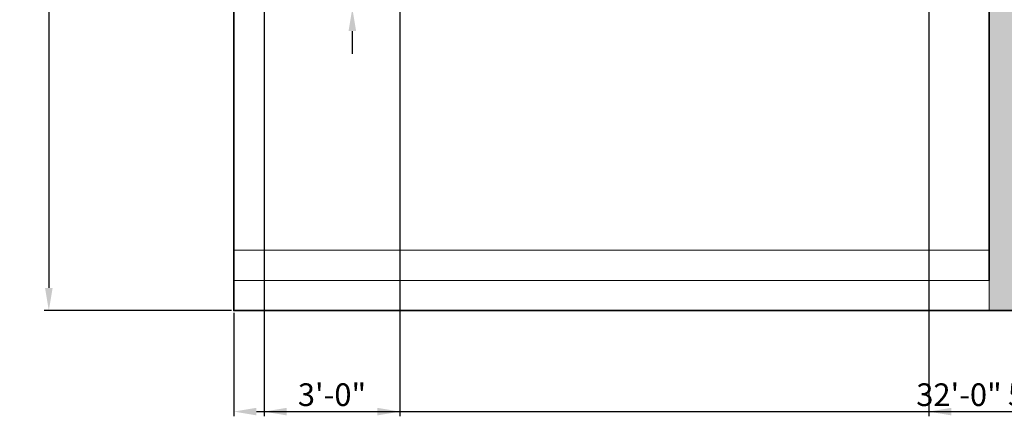
# Model space of a CAD drawing. Units: inches. Extents: x 2129 to 3258, y 1851 to 3021.
# Tile 1 of 10: x 2129 to 2390, y 1851 to 1956. Entities that reach past the tile are written whole.
import ezdxf

# ---------------------------------------------------------------- set-up
doc = ezdxf.new("R2010")
doc.units = ezdxf.units.IN
for name, color, linetype, lineweight in [('A-ANNO-DIMS', 2, 'Continuous', 18), ('A-FLOR-STRS', 7, 'Continuous', 20), ('A-WALL', 7, 'Continuous', 35)]:
    doc.layers.add(name, color=color, linetype=linetype, lineweight=lineweight)
doc.layers.add('A-WALL-PATT', color=32, linetype='Continuous', lineweight=13, true_color=0xcd6928)
doc.styles.get("Standard").update_dxf_attribs({"font": 'arial.ttf'})
doc.dimstyles.new('ISO-25', dxfattribs={"dimtxt": 6, "dimasz": 6, "dimexe": 1.25, "dimexo": 0.625, "dimtad": 1, "dimdec": 1, "dimlunit": 3, "dimtxsty": 'Standard', "dimcen": 2.5, "dimclrd": 5, "dimclre": 5, "dimadec": 0, "dimazin": 0, "dimtfac": 1, "dimtdec": 1, "dimtmove": 0, "dimatfit": 3, "dimfxl": 1, "dimarcsym": 0})

# ---------------------------------------------------------------- blocks, each defined once
blk = doc.blocks.new('*D6')
at = {"layer": 'A-ANNO-DIMS', "color": 0, "lineweight": -2, "transparency": 16777216}
for p, q in [((2185.3, 2407.23), (2135.71, 2407.23)), ((2136.96, 2401.23), (2136.96, 1885.23)), ((2185.3, 1879.23), (2135.71, 1879.23))]:
    blk.add_line(p, q, dxfattribs=at)
at = {"layer": 'A-ANNO-DIMS', "color": 0, "transparency": 16777216}
for points in [[(2135.96, 2401.23), (2137.96, 2401.23), (2136.96, 2407.23)], [(2135.96, 1885.23), (2137.96, 1885.23), (2136.96, 1879.23)]]:
    blk.add_solid(points, dxfattribs=at)
at = {"layer": 'Defpoints', "color": 0, "transparency": 16777216}
for p in [(2185.93, 2407.23), (2136.96, 1879.23), (2185.93, 1879.23)]:
    blk.add_point(p, dxfattribs=at)
at = {"layer": 'A-ANNO-DIMS', "color": 0, "transparency": 16777216, "insert": (2133.34, 2143.23), "char_height": 6, "attachment_point": 5, "rotation": 90}
blk.add_mtext("44'", dxfattribs=at)
blk = doc.blocks.new('*D63')
at = {"layer": 'A-ANNO-DIMS', "color": 5, "lineweight": -2, "transparency": 16777216}
for p, q in [((2217.31, 1973.23), (2217.31, 2017.06)), ((2221.94, 1967.23), (2216.06, 1967.23)), ((2217.31, 1959.23), (2217.31, 1967.23)), ((2221.94, 1959.23), (2216.06, 1959.23)), ((2217.31, 1953.23), (2217.31, 1947.23))]:
    blk.add_line(p, q, dxfattribs=at)
at = {"layer": 'A-ANNO-DIMS', "color": 5, "transparency": 16777216}
for points in [[(2216.31, 1973.23), (2218.31, 1973.23), (2217.31, 1967.23)], [(2216.31, 1953.23), (2218.31, 1953.23), (2217.31, 1959.23)]]:
    blk.add_solid(points, dxfattribs=at)
at = {"layer": 'Defpoints', "color": 0, "transparency": 16777216}
for p in [(2217.31, 1967.23), (2222.56, 1967.23), (2222.56, 1959.23)]:
    blk.add_point(p, dxfattribs=at)
at = {"layer": 'A-ANNO-DIMS', "color": 0, "transparency": 16777216, "insert": (2213.63, 1998.15), "char_height": 6, "attachment_point": 5, "rotation": 90}
blk.add_mtext('0\'-8" TYP.', dxfattribs=at)
blk = doc.blocks.new('*D86')
at = {"layer": 'A-ANNO-DIMS', "color": 5, "lineweight": -2, "transparency": 16777216}
for p, q in [((2185.93, 1878.61), (2185.93, 1851.23)), ((2569.93, 1878.61), (2569.93, 1851.23)), ((2191.93, 1852.48), (2563.93, 1852.48))]:
    blk.add_line(p, q, dxfattribs=at)
at = {"layer": 'A-ANNO-DIMS', "color": 5, "transparency": 16777216}
for points in [[(2191.93, 1853.48), (2191.93, 1851.48), (2185.93, 1852.48)], [(2563.93, 1853.48), (2563.93, 1851.48), (2569.93, 1852.48)]]:
    blk.add_solid(points, dxfattribs=at)
at = {"layer": 'Defpoints', "color": 0, "transparency": 16777216}
for p in [(2185.93, 1879.23), (2569.93, 1879.23), (2569.93, 1852.48)]:
    blk.add_point(p, dxfattribs=at)
at = {"layer": 'A-ANNO-DIMS', "color": 0, "transparency": 16777216, "insert": (2377.93, 1856.18), "char_height": 6, "attachment_point": 5}
blk.add_mtext('32\'-0"', dxfattribs=at)
blk = doc.blocks.new('*D91')
at = {"layer": 'A-ANNO-DIMS', "color": 5, "lineweight": -2, "transparency": 16777216}
for p, q in [((2369.93, 2314.61), (2369.93, 1851.23)), ((2429.93, 2314.61), (2429.93, 1851.23)), ((2375.93, 1852.48), (2423.93, 1852.48))]:
    blk.add_line(p, q, dxfattribs=at)
at = {"layer": 'A-ANNO-DIMS', "color": 5, "transparency": 16777216}
for points in [[(2375.93, 1853.48), (2375.93, 1851.48), (2369.93, 1852.48)], [(2423.93, 1853.48), (2423.93, 1851.48), (2429.93, 1852.48)]]:
    blk.add_solid(points, dxfattribs=at)
at = {"layer": 'Defpoints', "color": 0, "transparency": 16777216}
for p in [(2369.93, 2315.23), (2429.93, 2315.23), (2429.93, 1852.48)]:
    blk.add_point(p, dxfattribs=at)
at = {"layer": 'A-ANNO-DIMS', "color": 0, "transparency": 16777216, "insert": (2399.93, 1856.17), "char_height": 6, "attachment_point": 5}
blk.add_mtext('5\'-0"', dxfattribs=at)
blk = doc.blocks.new('*D97')
at = {"layer": 'A-ANNO-DIMS', "color": 5, "lineweight": -2, "transparency": 16777216}
for p, q in [((2193.93, 2272.48), (2193.93, 1851.23)), ((2229.93, 2272.48), (2229.93, 1851.23)), ((2199.93, 1852.48), (2223.93, 1852.48))]:
    blk.add_line(p, q, dxfattribs=at)
at = {"layer": 'A-ANNO-DIMS', "color": 5, "transparency": 16777216}
for points in [[(2199.93, 1853.48), (2199.93, 1851.48), (2193.93, 1852.48)], [(2223.93, 1853.48), (2223.93, 1851.48), (2229.93, 1852.48)]]:
    blk.add_solid(points, dxfattribs=at)
at = {"layer": 'Defpoints', "color": 0, "transparency": 16777216}
for p in [(2193.93, 2273.1), (2229.93, 2273.1), (2229.93, 1852.48)]:
    blk.add_point(p, dxfattribs=at)
at = {"layer": 'A-ANNO-DIMS', "color": 0, "transparency": 16777216, "insert": (2211.93, 1856.18), "char_height": 6, "attachment_point": 5}
blk.add_mtext('3\'-0"', dxfattribs=at)

msp = doc.modelspace()

# ---------------------------------------------------------------- hatches: boundary and pattern name
at = {"layer": 'A-WALL-PATT'}
h = msp.add_hatch(color=256, dxfattribs=at)
h.dxf.hatch_style = 1
h.paths.add_polyline_path([(2393.39, 2407.23), (2185.93, 2407.23), (2185.93, 2394.06), (2193.93, 2394.06), (2193.93, 2399.23), (2361.93, 2399.23), (2361.93, 2355.23), (2361.93, 2347.23), (2361.93, 2258.25), (2369.93, 2258.25), (2369.93, 2307.23), (2429.93, 2307.23), (2429.93, 2303.23), (2437.93, 2303.23), (2437.93, 2327.23), (2429.93, 2327.23), (2429.93, 2315.23), (2369.93, 2315.23), (2369.93, 2399.23), (2393.39, 2399.23)])
h.paths.add_polyline_path([(2569.93, 2407.23), (2410.42, 2407.23), (2410.42, 2399.23), (2429.93, 2399.23), (2429.93, 2351.23), (2437.93, 2351.23), (2437.93, 2399.23), (2561.93, 2399.23), (2561.93, 2317.22), (2569.93, 2317.22)])
h.paths.add_polyline_path([(2569.93, 2282.22), (2561.93, 2282.22), (2561.93, 2243.23), (2437.93, 2243.23), (2437.93, 2249.23), (2429.93, 2249.23), (2429.93, 2235.23), (2561.93, 2235.23), (2561.93, 2155.23), (2379.93, 2155.23), (2379.93, 2147.23), (2385.93, 2147.23), (2385.93, 2141.23), (2393.93, 2141.23), (2393.93, 2147.23), (2469.93, 2147.23), (2469.93, 2111.23), (2477.93, 2111.23), (2477.93, 2147.23), (2561.93, 2147.23), (2561.93, 2129.53), (2569.93, 2129.53)])
h.paths.add_polyline_path([(2569.93, 2112.5), (2561.93, 2112.5), (2561.93, 2063.23), (2477.93, 2063.23), (2477.93, 2069.23), (2469.93, 2069.23), (2469.93, 2063.23), (2445.93, 2063.23), (2445.93, 2055.23), (2561.93, 2055.23), (2561.93, 1951.04), (2569.93, 1951.04)])
h.paths.add_polyline_path([(2569.93, 1916.04), (2561.93, 1916.04), (2561.93, 1887.23), (2393.93, 1887.23), (2393.93, 2055.23), (2399.93, 2055.23), (2399.93, 2063.23), (2393.93, 2063.23), (2393.93, 2087.23), (2385.93, 2087.23), (2385.93, 1887.23), (2385.93, 1879.23), (2569.93, 1879.23)])
h.paths.add_polyline_path([(2193.93, 2147.23), (2289.93, 2147.23), (2289.93, 2155.23), (2193.93, 2155.23), (2193.93, 2170.77), (2185.93, 2170.77), (2185.93, 2056.85), (2193.93, 2056.85)])
h.paths.add_polyline_path([(2193.93, 2021.85), (2185.93, 2021.85), (2185.93, 1959.23), (2222.56, 1959.23), (2222.56, 1967.23), (2193.93, 1967.23)])
h.paths.add_polyline_path([(2307.93, 1967.23), (2257.56, 1967.23), (2257.56, 1959.23), (2307.93, 1959.23)])
h.paths.add_polyline_path([(2255.61, 2368.18), (2321.09, 2368.18), (2321.09, 2384.66), (2255.61, 2384.66)], flags=25)
h.paths.add_polyline_path([(2282.89, 2032.34), (2325.27, 2032.34), (2325.27, 2051.27), (2282.89, 2051.27)], flags=9)
h.paths.add_polyline_path([(2404.09, 1945.18), (2463.36, 1945.18), (2463.36, 1961.66), (2404.09, 1961.66)], flags=25)
h.paths.add_polyline_path([(2494.41, 2286.84), (2553.68, 2286.84), (2553.68, 2303.32), (2494.41, 2303.32)], flags=9)
h.paths.add_polyline_path([(2389.71, 2321.98), (2411.09, 2321.98), (2411.09, 2338.47), (2389.71, 2338.47)], flags=25)
h.paths.add_polyline_path([(2219.41, 2162.82), (2258.18, 2162.82), (2258.18, 2179.3), (2219.41, 2179.3)], flags=9)
h.paths.add_polyline_path([(2249.68, 2306.23), (2298.12, 2306.23), (2298.12, 2323.98), (2249.68, 2323.98)], flags=25)

# ---------------------------------------------------------------- linework, layer by layer
at = {"layer": 'A-FLOR-STRS'}
for p, q in [((2185.93, 1895.23), (2385.93, 1895.23)), ((2185.93, 1887.23), (2385.93, 1887.23)), ((2385.93, 1887.23), (2385.93, 1879.23))]:
    msp.add_line(p, q, dxfattribs=at)
msp.add_lwpolyline([(2385.93, 1887.23), (2193.93, 1887.23)], dxfattribs=at)
at = {"layer": 'A-WALL'}
msp.add_line((2385.93, 1887.23), (2385.93, 2087.23), dxfattribs=at)
msp.add_lwpolyline([(2185.93, 2407.23), (2569.93, 2407.23), (2569.93, 1879.23), (2185.93, 1879.23)], close=True, dxfattribs=at)

# ---------------------------------------------------------------- dimensions: what is measured, and where the dimension line sits
at = {"layer": 'A-ANNO-DIMS'}
dim = msp.add_linear_dim(base=(2136.96, 1879.23), p1=(2185.93, 2407.23), p2=(2185.93, 1879.23), angle=90, dimstyle='ISO-25', override={"dimclrd": 0, "dimclre": 0, "dimclrt": 0}, dxfattribs=at)
dim.commit()
dim.dimension.update_dxf_attribs({"geometry": '*D6', "text_midpoint": (2133.34, 2143.23)})
for base, p1, p2, picture, middle in [((2429.93, 1852.48), (2369.93, 2315.23), (2429.93, 2315.23), '*D91', (2399.93, 1856.17)), ((2229.93, 1852.48), (2193.93, 2273.1), (2229.93, 2273.1), '*D97', (2211.93, 1856.18)), ((2569.93, 1852.48), (2185.93, 1879.23), (2569.93, 1879.23), '*D86', (2377.93, 1856.18))]:
    dim = msp.add_linear_dim(base=base, p1=p1, p2=p2, dimstyle='ISO-25', override={"dimdec": 1, "dimlfac": 1, "dimrnd": 0, "dimzin": 1, "dimdsep": 46, "dimlunit": 4, "dimfrac": 2}, dxfattribs=at)
    dim.commit()
    dim.dimension.update_dxf_attribs({"geometry": picture, "text_midpoint": middle})
dim = msp.add_linear_dim(base=(2217.31, 1967.23), p1=(2222.56, 1959.23), p2=(2222.56, 1967.23), angle=90, text='<> TYP.', dimstyle='ISO-25', override={"dimdec": 1, "dimlfac": 1, "dimrnd": 0, "dimzin": 1, "dimdsep": 46, "dimlunit": 4, "dimfrac": 2}, dxfattribs=at)
dim.commit()
dim.dimension.update_dxf_attribs({"geometry": '*D63', "text_midpoint": (2213.63, 1998.15)})

doc.saveas('drawing.dxf')
